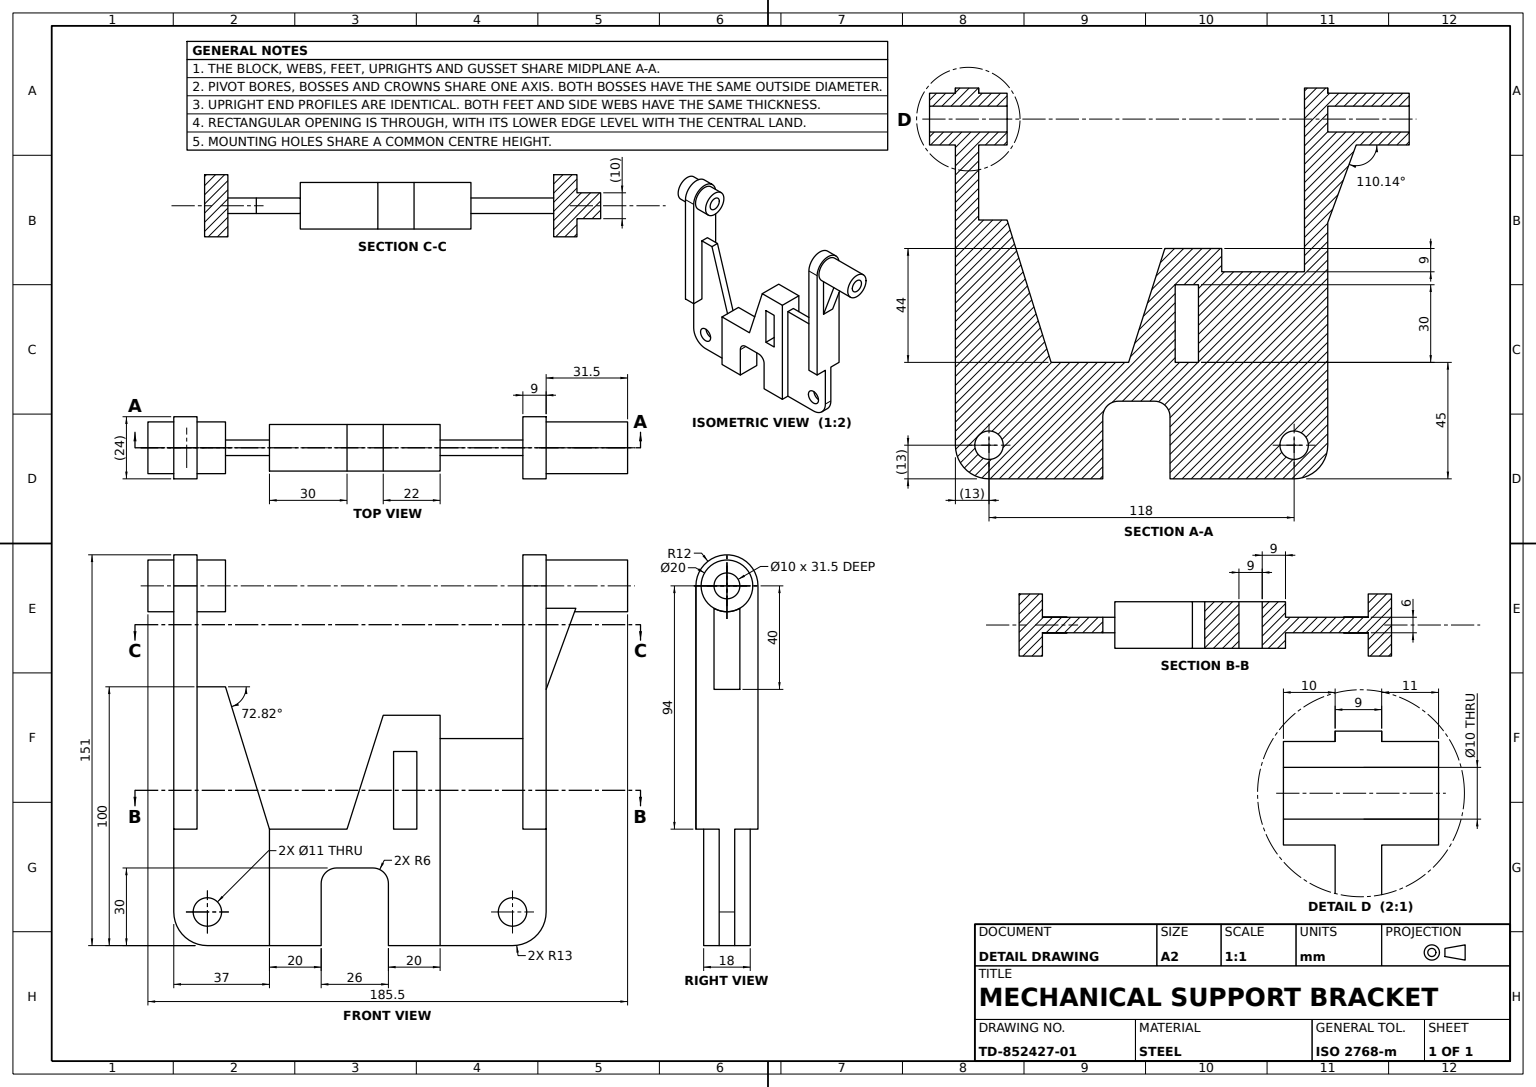
from build123d import *

# Parameters (mm, degrees)
BASE_PLATE_SKETCH_W            = 9
BASE_PLATE_SKETCH_H            = 30
BASE_PLATE_DEPTH               = 9
LEFT_ARM_SKETCH_R              = 5.5
LEFT_ARM_DEPTH                 = 3
LEFT_ARM_UPRIGHT_DEPTH         = 9
LEFT_PIVOT_BOSS_SKETCH_R       = 10
LEFT_PIVOT_BOSS_SKETCH_R_2     = 5
LEFT_PIVOT_BOSS_20_DEPTH       = 31.5
LEFT_GUSSET_RIB_REACH          = 186.595
LEFT_GUSSET_SKETCH_WALL_W      = 403.142743776
LEFT_GUSSET_SKETCH_WALL_H      = 10
RIGHT_ARM_SKETCH_R             = 5.5
RIGHT_ARM_DEPTH                = 3
RIGHT_START                    = -9
RIGHT_ARM_UPRIGHT_DEPTH        = 9
RIGHT_PIVOT_BOSS_20_DEPTH      = 10
RIGHT_PIVOT_BOSS_20_DEPTH_BACK = 20
RIGHT_PIVOT_BOSS_SKETCH_R      = 10
RIGHT_PIVOT_BOSS_SKETCH_R_2    = 5
PIVOT_START                    = -38
PIVOT_CUT_SKETCH_R             = 5
PIVOT_CUT_DEPTH                = 38


with BuildPart() as part:
    # Base Plate Sketch → Base Plate (new, symmetric)
    with BuildSketch(Plane.XY):
        with BuildLine():
            Line((-7, 30), (7, 30))
            ThreePointArc((7, 30), (11.242640687, 28.242640687), (13, 24))
            Line((13, 24), (13, 0))
            Line((13, 0), (33, 0))
            Line((33, 0), (33, 89))
            Line((33, 89), (11, 89))
            Line((11, 89), (-3, 45))
            Line((-3, 45), (-33, 45))
            Line((-33, 45), (-33, 0))
            Line((-33, 0), (-13, 0))
            Line((-13, 0), (-13, 24))
            ThreePointArc((-13, 24), (-11.242640687, 28.242640687), (-7, 30))
        make_face()
        with Locations((19.5, 60)):
            Rectangle(BASE_PLATE_SKETCH_W, BASE_PLATE_SKETCH_H, mode=Mode.SUBTRACT)
    extrude(amount=BASE_PLATE_DEPTH, both=True)

    # Left Arm Sketch → Left Arm (add, symmetric)
    with BuildSketch(Plane.XY):
        with BuildLine():
            Line((33, 0), (61, 0))
            ThreePointArc((61, 0), (70.192388155, 3.807611845), (74, 13))
            Line((74, 13), (74, 80))
            Line((74, 80), (33, 80))
            Line((33, 80), (33, 0))
        make_face()
        with Locations((61, 13)):
            Circle(LEFT_ARM_SKETCH_R, mode=Mode.SUBTRACT)
    extrude(amount=LEFT_ARM_DEPTH, both=True)

    # Left Arm Upright Sketch → Left Arm Upright (add)
    with BuildSketch(Plane(origin=(74, 0, 0), x_dir=(0, 0, -1), z_dir=(1, 0, 0))):
        with BuildLine():
            Line((-12, 45), (12, 45))
            Line((12, 45), (12, 139))
            ThreePointArc((12, 139), (0, 151), (-12, 139))
            Line((-12, 139), (-12, 45))
        make_face()
    extrude(amount=-LEFT_ARM_UPRIGHT_DEPTH)

    # Left Pivot Boss Sketch → Left Pivot Boss Ø20 (add)
    with BuildSketch(Plane(origin=(74, 0, 0), x_dir=(0, 0, -1), z_dir=(1, 0, 0))):
        with Locations(Location((0, 139, 0), (0, 0, 180))):
            Circle(LEFT_PIVOT_BOSS_SKETCH_R)
        with Locations((0, 139)):
            Circle(LEFT_PIVOT_BOSS_SKETCH_R_2, mode=Mode.SUBTRACT)
    extrude(amount=LEFT_PIVOT_BOSS_20_DEPTH)

    # Left Gusset Sketch wall → Left Gusset Rib (add, up to next)
    with BuildSketch(Plane(origin=(79.5, 114, 0), x_dir=(-0.344254649158, -0.938876315887, 0), z_dir=(0.938876315887, -0.344254649158, 0)), mode=Mode.PRIVATE) as left_gusset_rib_sk1:
        Rectangle(LEFT_GUSSET_SKETCH_WALL_W, LEFT_GUSSET_SKETCH_WALL_H)
    left_gusset_rib_tool1 = extrude(left_gusset_rib_sk1.sketch, amount=-LEFT_GUSSET_RIB_REACH, mode=Mode.PRIVATE) - part.part
    add(left_gusset_rib_tool1.solids().sort_by_distance((79.5, 114, 0))[0])

    # Right Arm Sketch → Right Arm (add, symmetric)
    with BuildSketch(Plane.XY):
        with BuildLine():
            Line((-33, 0), (-57, 0))
            ThreePointArc((-57, 0), (-66.192388155, 3.807611845), (-70, 13))
            Line((-70, 13), (-70, 100))
            Line((-70, 100), (-50, 100))
            Line((-50, 100), (-33, 45))
            Line((-33, 45), (-33, 0))
        make_face()
        with Locations((-57, 13)):
            Circle(RIGHT_ARM_SKETCH_R, mode=Mode.SUBTRACT)
    extrude(amount=RIGHT_ARM_DEPTH, both=True)

    # Right Arm Upright Sketch → Right Arm Upright (add)
    with BuildSketch(Plane.ZY.offset(70).offset(RIGHT_START)):
        with BuildLine():
            Line((12, 45), (-12, 45))
            Line((-12, 45), (-12, 139))
            ThreePointArc((-12, 139), (0, 151), (12, 139))
            Line((12, 139), (12, 45))
        make_face()
    extrude(amount=RIGHT_ARM_UPRIGHT_DEPTH)

    # Right Pivot Boss Sketch → Right Pivot Boss Ø20 (add, two sides: drawn at the far end of the back side and taken through both)
    with BuildSketch(Plane.ZY.offset(70).offset(-RIGHT_PIVOT_BOSS_20_DEPTH_BACK)):
        with Locations(Location((0, 139, 0), (0, 0, 300))):
            Circle(RIGHT_PIVOT_BOSS_SKETCH_R)
        with Locations(Location((0, 139, 0), (0, 0, 180))):
            Circle(RIGHT_PIVOT_BOSS_SKETCH_R_2, mode=Mode.SUBTRACT)
    extrude(amount=RIGHT_PIVOT_BOSS_20_DEPTH + RIGHT_PIVOT_BOSS_20_DEPTH_BACK)

    # Pivot Cut Sketch → Pivot Cut (cut)
    with BuildSketch(Plane(origin=(-50, 0, 0), x_dir=(0, 0, -1), z_dir=(1, 0, 0)).offset(PIVOT_START)):
        with Locations((0, 139)):
            Circle(PIVOT_CUT_SKETCH_R)
    extrude(amount=PIVOT_CUT_DEPTH, mode=Mode.SUBTRACT)


solid = part.part
